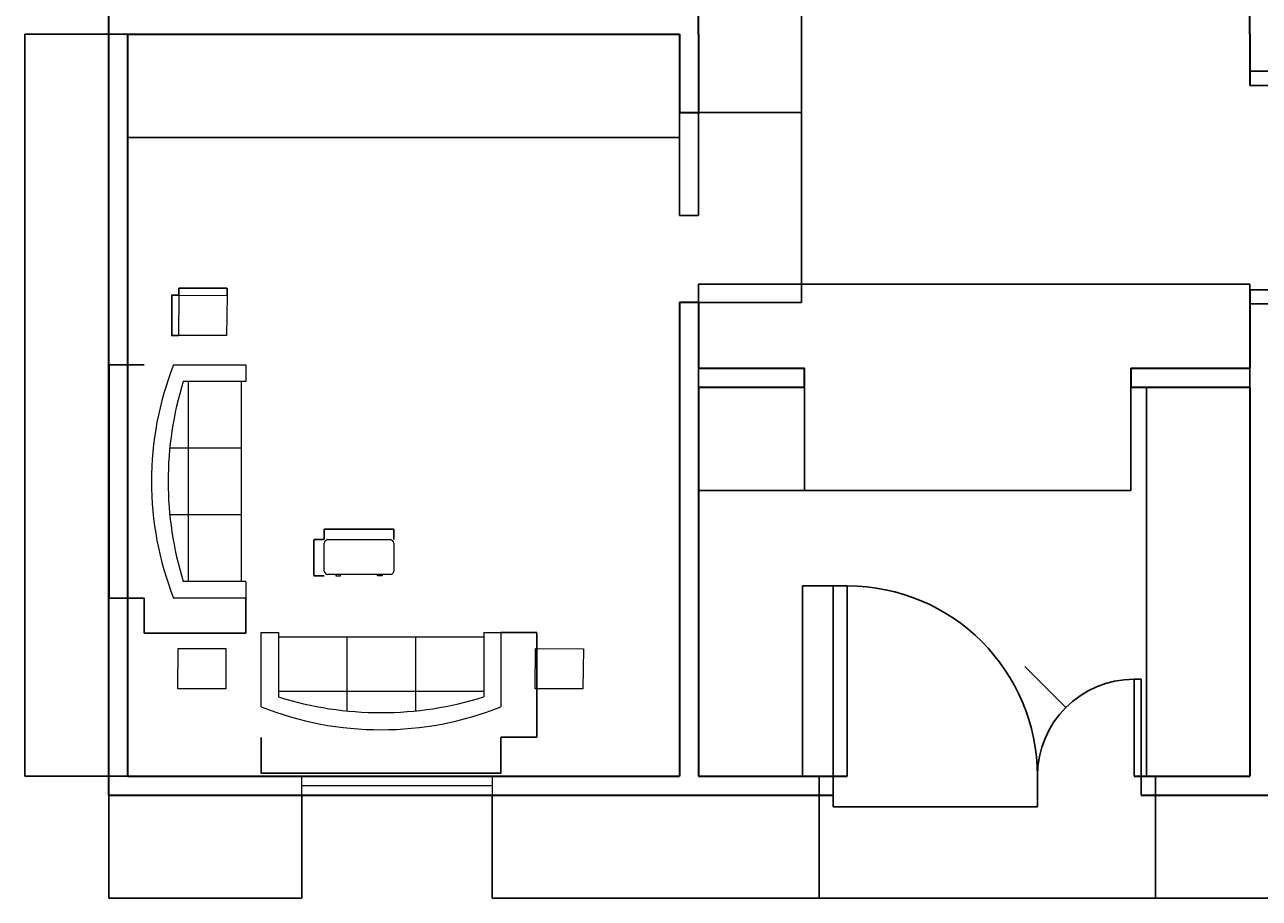
# Model space of a CAD drawing. Units: millimetres. Extents: x 1426 to 11512, y -8522 to 2664.
# Tile 1 of 4: x 1426 to 7919, y -8522 to -3929. Entities that reach past the tile are written whole.
import ezdxf

# ---------------------------------------------------------------- set-up
doc = ezdxf.new("R2010")
doc.units = ezdxf.units.MM
for name, color, linetype, lineweight in [('A-ANNO-DIMS', 2, 'Continuous', 18), ('A-DOOR', 3, 'Continuous', 25), ('A-FURN', 8, 'Continuous', 18), ('A-GLAZ', 4, 'Continuous', 18), ('A-WALL', 7, 'Continuous', 35)]:
    doc.layers.add(name, color=color, linetype=linetype, lineweight=lineweight)
doc.styles.get("Standard").update_dxf_attribs({"font": 'arial.ttf'})
doc.dimstyles.get("Standard").update_dxf_attribs({"dimtxt": 0.18, "dimasz": 0.18, "dimexe": 0.18, "dimexo": 0.0625, "dimgap": 0.09, "dimtad": 0, "dimtih": 1, "dimtoh": 1, "dimdec": 4, "dimzin": 0, "dimdsep": 46, "dimtxsty": 'Standard', "dimcen": 0.09, "dimadec": 0, "dimazin": 0, "dimtfac": 1, "dimtdec": 4, "dimtofl": 0, "dimtmove": 0, "dimatfit": 3, "dimfxl": 1, "dimtolj": 1, "dimtzin": 0, "dimarcsym": 0})

# ---------------------------------------------------------------- blocks, each defined once
blk = doc.blocks.new('Sofa - Roundback 7 ft.')
for p, q in [((-12.00002, -32.44210000000393), (-12.00003, -6.597100000003898)), ((11.99996999999999, -32.44210000000393), (11.99997999999999, -6.597100000003898)), ((-36.000027, -34.00000000000395), (-36.000027, -11.46960000000396)), ((35.99997999999999, -34.00000000000395), (35.99997999999999, -11.46960000000396)), ((-35.999844, -13.38190000000397), (35.99979999999999, -13.38190000000397)), ((-36.000027, -32.44210000000393), (35.99997999999999, -32.44210000000393))]:
    blk.add_line(p, q)
for points in [[(-36.000027, -34.00000000000395), (-42.000027, -34.00000000000395), (-42.000027, -8.000000000003944)], [(41.99997999999999, -8.000000000003944), (41.99997999999999, -34.00000000000395), (35.99997999999999, -34.00000000000395)]]:
    blk.add_lwpolyline(points)
for centre, radius, start, end in [((0, -114.2500000000039), 114.2500000000039, 68.43141000000072, 111.5686000000006), ((-1.00000000032e-05, -127.1968000000039), 121.1967999999973, 72.72032999999948, 107.2797000000005)]:
    blk.add_arc(centre, radius, start, end)
blk = doc.blocks.new('Desk - 30 x 60 in.')
for p, q in [((-26.999995, 0), (26.999995, 0)), ((-29.999995, -27), (-29.999995, -3)), ((29.999995, -3), (29.999995, -27)), ((26.999995, -30), (-26.999995, -30)), ((-20.000005, -30), (-20.000005, -31)), ((-20.000005, -31), (-16.000005, -31)), ((-16.000005, -31), (-16.000005, -30)), ((15.999995, -31), (15.999995, -30)), ((19.999995, -31), (15.999995, -31)), ((19.999995, -30), (19.999995, -31))]:
    blk.add_line(p, q)
for centre, radius, start, end in [((-26.499995, -3.5), 3.535534000004229, 98.1300999999916, 171.8698999999352), ((26.499995, -3.5), 3.535533999997753, 8.130102000022115, 81.8698999999439), ((-26.499995, -26.5), 3.535534000000845, 188.1301000000653, 261.8699000000085), ((26.499995, -26.5), 3.535534000004826, 278.1301000000561, 351.8698999999439)]:
    blk.add_arc(centre, radius, start, end)
blk = doc.blocks.new('DOOR-SINGLE-1000')
for p, q in [((-0.0002449408875691, 999.9999577541435), (-0.0002449408875691, 1099.999957754143)), ((-0.0002449408875691, 1099.999957754143), (74.19975505911316, 1099.999957754143)), ((74.19975505911316, 1099.999957754143), (74.19975505911316, 999.9999577541435)), ((1148.399755059116, 999.999957754143), (1148.399755059116, 1099.999957754143)), ((1148.399755059116, 1099.999957754143), (1222.599755059116, 1099.999957754143)), ((1222.599755059116, 1099.999957754143), (1222.599755059116, 999.9999577541435)), ((74.19975505911316, 999.9999577541435), (-0.0002449408875691, 999.9999577541435)), ((74.19975505911316, 999.9999577541435), (148.3997550591139, 999.9999577541435)), ((74.19975505911316, -4.22458564344e-05), (74.19975505911316, 999.9999577541435)), ((148.3997550591139, 999.9999577541435), (148.3997550591139, -4.22458564344e-05)), ((1222.599755059116, 999.999957754143), (1148.399755059116, 999.999957754143)), ((148.3997550591139, -4.22458564344e-05), (74.19975505911316, -4.22458564344e-05))]:
    blk.add_line(p, q)
blk.add_arc((148.3997550591157, 999.9999577541435), 999.9999999999998, 270, 0)
blk = doc.blocks.new('DOOR-LEAF-1000')
for p, q in [((999.9997662421769, 74.19984207478274), (-0.0002337578230254, 74.19984207478274)), ((-0.0002337578230254, 74.19984207478274), (-0.0002337578230254, -0.0001579252179909)), ((999.9997662421769, -0.0001579252179909), (999.9997662421769, 74.19984207478274)), ((-0.0002337578230254, -0.0001579252179909), (999.9997662421769, -0.0001579252179909))]:
    blk.add_line(p, q)
blk.add_arc((999.9997662421769, 74.19984207478456), 999.9999999999998, 90, 180)
blk = doc.blocks.new('WIN-1000')
for p, q in [((-0.0003881192678818, 99.99995775414573), (999.999611880732, 99.99995775414573)), ((-0.0003881192678818, -4.22458542744e-05), (-0.0003881192678818, 99.99995775414573)), ((999.999611880732, 99.99995775414573), (999.999611880732, -4.22458542744e-05)), ((-0.0003881192678818, 49.99995775414572), (999.999611880732, 49.99995775414572)), ((999.999611880732, -4.22458542744e-05), (-0.0003881192678818, -4.22458542744e-05))]:
    blk.add_line(p, q)
blk = doc.blocks.new('TABLE-END')
for p, q in [((0.5765397481395667, 0.4802073471801123), (1.381469779128565, 211.490897786076)), ((1.381469779128565, 211.490897786076), (253.6387314006142, 210.5286268935834)), ((253.6387314006142, 210.5286268935834), (250.8785212126982, -0.4746048534607326)), ((250.8785212126982, -0.4746048534607326), (0.5765397481395667, 0.4802073471801123))]:
    blk.add_line(p, q)
blk = doc.blocks.new('*D16')
at = {"layer": 'A-ANNO-DIMS', "color": 0, "lineweight": -2, "transparency": 16777216}
for p, q in [((2237.041557626602, -5351.488836398402), (2237.041557626602, -5313.41200765053)), ((2237.221557626601, -5313.59200765053), (2362.245736672484, -5313.59200765053)), ((2489.923749279077, -5313.59200765053), (2364.899570233193, -5313.59200765053)), ((2490.103749279076, -5351.488836398402), (2490.103749279076, -5313.41200765053))]:
    blk.add_line(p, q, dxfattribs=at)
at = {"layer": 'A-ANNO-DIMS', "color": 0, "transparency": 16777216}
for points in [[(2237.221557626601, -5313.562007650531), (2237.221557626601, -5313.622007650531), (2237.041557626602, -5313.59200765053)], [(2489.923749279077, -5313.562007650531), (2489.923749279077, -5313.622007650531), (2490.103749279076, -5313.59200765053)]]:
    blk.add_solid(points, dxfattribs=at)
at = {"layer": 'Defpoints', "color": 0, "transparency": 16777216}
for p in [(2490.103749279076, -5313.59200765053), (2237.041557626602, -5351.551336398402), (2490.103749279076, -5351.551336398402)]:
    blk.add_point(p, dxfattribs=at)
at = {"layer": 'A-ANNO-DIMS', "color": 0, "transparency": 16777216, "insert": (2363.572653452838, -5313.59200765053), "char_height": 0.18, "attachment_point": 5}
blk.add_mtext('\\A1;END TABLE 253 TYP.', dxfattribs=at)
blk = doc.blocks.new('*D17')
at = {"layer": 'A-ANNO-DIMS', "color": 0, "lineweight": -2, "transparency": 16777216}
for p, q in [((2236.979057626602, -5351.551336398404), (2198.902228878733, -5351.551336398404)), ((2199.082228878732, -5351.731336398405), (2199.082228878732, -5457.35365797738)), ((2199.082228878732, -5563.33683903794), (2199.082228878732, -5457.714517458963)), ((2236.979057626602, -5563.516839037941), (2198.902228878733, -5563.516839037941))]:
    blk.add_line(p, q, dxfattribs=at)
at = {"layer": 'A-ANNO-DIMS', "color": 0, "transparency": 16777216}
for points in [[(2199.052228878732, -5351.731336398405), (2199.112228878732, -5351.731336398405), (2199.082228878732, -5351.551336398404)], [(2199.052228878732, -5563.33683903794), (2199.112228878732, -5563.33683903794), (2199.082228878732, -5563.516839037941)]]:
    blk.add_solid(points, dxfattribs=at)
at = {"layer": 'Defpoints', "color": 0, "transparency": 16777216}
for p in [(2199.082228878732, -5351.551336398404), (2237.041557626602, -5351.551336398404), (2237.041557626602, -5563.516839037941)]:
    blk.add_point(p, dxfattribs=at)
at = {"layer": 'A-ANNO-DIMS', "color": 0, "transparency": 16777216, "insert": (2199.08222887873, -5457.534087718172), "char_height": 0.18, "attachment_point": 5}
blk.add_mtext('\\A1;212 TYP.', dxfattribs=at)
blk = doc.blocks.new('*D18')
at = {"layer": 'A-ANNO-DIMS', "color": 0, "lineweight": -2, "transparency": 16777216}
for p, q in [((2053.688910879819, -5716.972741680017), (1869.607763812478, -5716.972741680017)), ((1869.787763812478, -5717.152741680017), (1869.787763812478, -6330.001767602539)), ((1869.787763812478, -6943.217055462304), (1869.787763812478, -6330.368029539783)), ((2053.688910879819, -6943.397055462305), (1869.607763812478, -6943.397055462305))]:
    blk.add_line(p, q, dxfattribs=at)
at = {"layer": 'A-ANNO-DIMS', "color": 0, "transparency": 16777216}
for points in [[(1869.757763812478, -5717.152741680017), (1869.817763812478, -5717.152741680017), (1869.787763812478, -5716.972741680017)], [(1869.757763812478, -6943.217055462304), (1869.817763812478, -6943.217055462304), (1869.787763812478, -6943.397055462305)]]:
    blk.add_solid(points, dxfattribs=at)
at = {"layer": 'Defpoints', "color": 0, "transparency": 16777216}
for p in [(1869.787763812478, -5716.972741680017), (2053.751410879819, -5716.972741680017), (2053.751410879819, -6943.397055462305)]:
    blk.add_point(p, dxfattribs=at)
at = {"layer": 'A-ANNO-DIMS', "color": 0, "transparency": 16777216, "insert": (1869.787763812475, -6330.184898571159), "char_height": 0.18, "attachment_point": 5}
blk.add_mtext('\\A1;SOFA 1226', dxfattribs=at)
blk = doc.blocks.new('*D19')
at = {"layer": 'A-ANNO-DIMS', "color": 0, "lineweight": -2, "transparency": 16777216}
for p, q in [((2053.751410879818, -6943.4595554623), (2053.751410879818, -7127.540702529643)), ((2589.095269586896, -6943.4595554623), (2589.095269586896, -7127.540702529643)), ((2053.931410879818, -7127.360702529642), (2321.133817723125, -7127.360702529642)), ((2588.915269586896, -7127.360702529642), (2321.712862743589, -7127.360702529642))]:
    blk.add_line(p, q, dxfattribs=at)
at = {"layer": 'A-ANNO-DIMS', "color": 0, "transparency": 16777216}
for points in [[(2053.931410879818, -7127.330702529643), (2053.931410879818, -7127.390702529644), (2053.751410879818, -7127.360702529642)], [(2588.915269586896, -7127.330702529643), (2588.915269586896, -7127.390702529644), (2589.095269586896, -7127.360702529642)]]:
    blk.add_solid(points, dxfattribs=at)
at = {"layer": 'Defpoints', "color": 0, "transparency": 16777216}
for p in [(2053.751410879818, -6943.3970554623), (2589.095269586896, -6943.3970554623), (2053.751410879818, -7127.360702529642)]:
    blk.add_point(p, dxfattribs=at)
at = {"layer": 'A-ANNO-DIMS', "color": 0, "transparency": 16777216, "insert": (2321.423340233357, -7127.360702529642), "char_height": 0.18, "attachment_point": 5}
blk.add_mtext('\\A1;535', dxfattribs=at)
blk = doc.blocks.new('*D20')
at = {"layer": 'A-ANNO-DIMS', "color": 0, "lineweight": -2, "transparency": 16777216}
for p, q in [((2670.058380604727, -7675.536986969425), (2670.058380604727, -7864.771040374122)), ((3930.835403302701, -7675.536986969425), (3930.835403302701, -7864.771040374122)), ((2670.238380604727, -7864.591040374121), (3299.728672308421, -7864.591040374121)), ((3930.655403302701, -7864.591040374121), (3301.165111599007, -7864.591040374121))]:
    blk.add_line(p, q, dxfattribs=at)
at = {"layer": 'A-ANNO-DIMS', "color": 0, "transparency": 16777216}
for points in [[(2670.238380604727, -7864.561040374121), (2670.238380604727, -7864.621040374121), (2670.058380604727, -7864.591040374121)], [(3930.655403302701, -7864.561040374121), (3930.655403302701, -7864.621040374121), (3930.835403302701, -7864.591040374121)]]:
    blk.add_solid(points, dxfattribs=at)
at = {"layer": 'Defpoints', "color": 0, "transparency": 16777216}
for p in [(2670.058380604727, -7675.474486969425), (3930.835403302701, -7675.474486969425), (2670.058380604727, -7864.591040374121)]:
    blk.add_point(p, dxfattribs=at)
at = {"layer": 'A-ANNO-DIMS', "color": 0, "transparency": 16777216, "insert": (3300.446891953714, -7864.591040374121), "char_height": 0.18, "attachment_point": 5}
blk.add_mtext('\\A1;SOFA 1261', dxfattribs=at)
blk = doc.blocks.new('*D21')
at = {"layer": 'A-ANNO-DIMS', "color": 0, "lineweight": -2, "transparency": 16777216}
for p, q in [((3930.897903302703, -7125.13540063901), (4120.131956707401, -7125.13540063901)), ((4119.9519567074, -7125.31540063901), (4119.9519567074, -7400.123040666429)), ((4119.9519567074, -7675.294486969429), (4119.9519567074, -7400.486846942008)), ((3930.897903302703, -7675.474486969429), (4120.131956707401, -7675.474486969429))]:
    blk.add_line(p, q, dxfattribs=at)
at = {"layer": 'A-ANNO-DIMS', "color": 0, "transparency": 16777216}
for points in [[(4119.9219567074, -7125.31540063901), (4119.9819567074, -7125.31540063901), (4119.9519567074, -7125.13540063901)], [(4119.9219567074, -7675.294486969429), (4119.9819567074, -7675.294486969429), (4119.9519567074, -7675.474486969429)]]:
    blk.add_solid(points, dxfattribs=at)
at = {"layer": 'Defpoints', "color": 0, "transparency": 16777216}
for p in [(3930.835403302703, -7125.13540063901), (3930.835403302703, -7675.474486969429), (4119.9519567074, -7675.474486969429)]:
    blk.add_point(p, dxfattribs=at)
at = {"layer": 'A-ANNO-DIMS', "color": 0, "transparency": 16777216, "insert": (4119.951956707398, -7400.304943804218), "char_height": 0.18, "attachment_point": 5}
blk.add_mtext('\\A1;550', dxfattribs=at)
blk = doc.blocks.new('*D26')
at = {"layer": 'A-ANNO-DIMS', "color": 0, "lineweight": -2, "transparency": 16777216}
for p, q in [((5677.730172282599, -7879.117542245857), (5677.730172282599, -8040.365042245856)), ((6751.930172282602, -7879.117542245857), (6751.930172282602, -8040.365042245856)), ((5677.910172282599, -8040.185042245855), (6213.405213210294, -8040.185042245855)), ((6751.750172282601, -8040.185042245855), (6216.255131354905, -8040.185042245855))]:
    blk.add_line(p, q, dxfattribs=at)
at = {"layer": 'A-ANNO-DIMS', "color": 0, "transparency": 16777216}
for points in [[(5677.910172282599, -8040.155042245855), (5677.910172282599, -8040.215042245856), (5677.730172282599, -8040.185042245855)], [(6751.750172282601, -8040.155042245855), (6751.750172282601, -8040.215042245856), (6751.930172282602, -8040.185042245855)]]:
    blk.add_solid(points, dxfattribs=at)
at = {"layer": 'Defpoints', "color": 0, "transparency": 16777216}
for p in [(5677.730172282599, -7879.055042245856), (6751.930172282602, -7879.055042245856), (6751.930172282602, -8040.185042245855)]:
    blk.add_point(p, dxfattribs=at)
at = {"layer": 'A-ANNO-DIMS', "color": 0, "transparency": 16777216, "insert": (6214.830172282599, -8040.185042245855), "char_height": 0.18, "attachment_point": 5}
blk.add_mtext('\\A1;DOOR LEAF 1074 TYP.', dxfattribs=at)
blk = doc.blocks.new('*D27')
at = {"layer": 'A-ANNO-DIMS', "color": 0, "lineweight": -2, "transparency": 16777216}
for p, q in [((5677.667672282598, -6879.055042245861), (5516.420172282601, -6879.055042245861)), ((5516.600172282601, -6879.235042245861), (5516.600172282601, -7378.87313910807)), ((5516.600172282601, -7878.87504224586), (5516.600172282601, -7379.23694538365)), ((5677.6676722826, -7879.055042245861), (5516.420172282601, -7879.055042245861))]:
    blk.add_line(p, q, dxfattribs=at)
at = {"layer": 'A-ANNO-DIMS', "color": 0, "transparency": 16777216}
for points in [[(5516.570172282602, -6879.235042245861), (5516.630172282601, -6879.235042245861), (5516.600172282601, -6879.055042245861)], [(5516.570172282602, -7878.87504224586), (5516.630172282601, -7878.87504224586), (5516.600172282601, -7879.055042245861)]]:
    blk.add_solid(points, dxfattribs=at)
at = {"layer": 'Defpoints', "color": 0, "transparency": 16777216}
for p in [(5677.730172282599, -6879.055042245861), (5516.600172282601, -7879.055042245861), (5677.730172282601, -7879.055042245861)]:
    blk.add_point(p, dxfattribs=at)
at = {"layer": 'A-ANNO-DIMS', "color": 0, "transparency": 16777216, "insert": (5516.600172282599, -7379.055042245859), "char_height": 0.18, "attachment_point": 5}
blk.add_mtext('\\A1;1000 TYP.', dxfattribs=at)
blk = doc.blocks.new('*D36')
at = {"layer": 'A-ANNO-DIMS', "color": 0, "lineweight": -2, "transparency": 16777216}
for p, q in [((3001.124611822948, -6636.252036484484), (3001.124611822948, -6581.182263887985)), ((3001.304611822947, -6581.362263887985), (3183.637237167347, -6581.362263887985)), ((3367.293095799605, -6581.362263887985), (3184.960470455205, -6581.362263887985)), ((3367.473095799605, -6636.252036484484), (3367.473095799605, -6581.182263887985))]:
    blk.add_line(p, q, dxfattribs=at)
at = {"layer": 'A-ANNO-DIMS', "color": 0, "transparency": 16777216}
for points in [[(3001.304611822947, -6581.332263887985), (3001.304611822947, -6581.392263887984), (3001.124611822948, -6581.362263887985)], [(3367.293095799605, -6581.332263887985), (3367.293095799605, -6581.392263887984), (3367.473095799605, -6581.362263887985)]]:
    blk.add_solid(points, dxfattribs=at)
at = {"layer": 'Defpoints', "color": 0, "transparency": 16777216}
for p in [(3367.473095799605, -6581.362263887985), (3001.124611822948, -6636.314536484483), (3367.473095799605, -6636.314536484483)]:
    blk.add_point(p, dxfattribs=at)
at = {"layer": 'A-ANNO-DIMS', "color": 0, "transparency": 16777216, "insert": (3184.298853811276, -6581.362263887985), "char_height": 0.18, "attachment_point": 5}
blk.add_mtext('\\A1;DESK 366', dxfattribs=at)
blk = doc.blocks.new('*D37')
at = {"layer": 'A-ANNO-DIMS', "color": 0, "lineweight": -2, "transparency": 16777216}
for p, q in [((3001.062111822948, -6636.314536484488), (2945.992339226451, -6636.314536484488)), ((2946.172339226451, -6636.494536484488), (2946.172339226451, -6730.772674135775)), ((2946.172339226451, -6825.414618062641), (2946.172339226451, -6731.136480411355)), ((3001.062111822948, -6825.594618062641), (2945.992339226451, -6825.594618062641))]:
    blk.add_line(p, q, dxfattribs=at)
at = {"layer": 'A-ANNO-DIMS', "color": 0, "transparency": 16777216}
for points in [[(2946.142339226451, -6636.494536484488), (2946.202339226451, -6636.494536484488), (2946.172339226451, -6636.314536484488)], [(2946.142339226451, -6825.414618062641), (2946.202339226451, -6825.414618062641), (2946.172339226451, -6825.594618062641)]]:
    blk.add_solid(points, dxfattribs=at)
at = {"layer": 'Defpoints', "color": 0, "transparency": 16777216}
for p in [(2946.172339226451, -6636.314536484488), (3001.124611822949, -6636.314536484488), (3001.124611822949, -6825.594618062641)]:
    blk.add_point(p, dxfattribs=at)
at = {"layer": 'A-ANNO-DIMS', "color": 0, "transparency": 16777216, "insert": (2946.172339226448, -6730.954577273563), "char_height": 0.18, "attachment_point": 5}
blk.add_mtext('\\A1;189', dxfattribs=at)
blk = doc.blocks.new('*D40')
at = {"layer": 'A-ANNO-DIMS', "color": 0, "lineweight": -2, "transparency": 16777216}
for p, q in [((1968.871984, -3979.117542), (1968.871984, -4521.735042)), ((4868.871984, -3979.117542), (4868.871984, -4521.735042)), ((1969.051984, -4521.555042), (3418.511984000001, -4521.555042)), ((4868.691984, -4521.555042), (3419.231984, -4521.555042))]:
    blk.add_line(p, q, dxfattribs=at)
at = {"layer": 'A-ANNO-DIMS', "color": 0, "transparency": 16777216}
for points in [[(1969.051984, -4521.525042), (1969.051984, -4521.585041999999), (1968.871984, -4521.555042)], [(4868.691984, -4521.525042), (4868.691984, -4521.585041999999), (4868.871984, -4521.555042)]]:
    blk.add_solid(points, dxfattribs=at)
at = {"layer": 'Defpoints', "color": 0, "transparency": 16777216}
for p in [(1968.871984, -3979.055042), (4868.871984, -3979.055042), (1968.871984, -4521.555042)]:
    blk.add_point(p, dxfattribs=at)
at = {"layer": 'A-ANNO-DIMS', "color": 0, "transparency": 16777216, "insert": (3418.871984000001, -4521.555042), "char_height": 0.18, "attachment_point": 5}
blk.add_mtext('\\A1;2900', dxfattribs=at)
blk = doc.blocks.new('*D41')
at = {"layer": 'A-ANNO-DIMS', "color": 0, "lineweight": -2, "transparency": 16777216}
for p, q in [((4968.871984, -5835.356649000001), (4968.871984, -5292.739148999999)), ((4969.051984, -5292.919149), (6418.511984000002, -5292.919149)), ((7868.691984, -5292.919149), (6419.231983999999, -5292.919149)), ((7868.871984, -5835.356649000001), (7868.871984, -5292.739148999999))]:
    blk.add_line(p, q, dxfattribs=at)
at = {"layer": 'A-ANNO-DIMS', "color": 0, "transparency": 16777216}
for points in [[(4969.051984, -5292.889149), (4969.051984, -5292.949149), (4968.871984, -5292.919149)], [(7868.691984, -5292.889149), (7868.691984, -5292.949149), (7868.871984, -5292.919149)]]:
    blk.add_solid(points, dxfattribs=at)
at = {"layer": 'Defpoints', "color": 0, "transparency": 16777216}
for p in [(7868.871984, -5292.919149), (4968.871984, -5835.419149), (7868.871984, -5835.419149)]:
    blk.add_point(p, dxfattribs=at)
at = {"layer": 'A-ANNO-DIMS', "color": 0, "transparency": 16777216, "insert": (6418.871984, -5292.919149), "char_height": 0.18, "attachment_point": 5}
blk.add_mtext('\\A1;2900', dxfattribs=at)
blk = doc.blocks.new('*D45')
at = {"layer": 'A-ANNO-DIMS', "color": 0, "lineweight": -2, "transparency": 16777216}
for p, q in [((1968.809484000001, -3979.055042000002), (1426.191984, -3979.055042000002)), ((1426.371984, -3979.235042000002), (1426.371984000001, -5928.873077470671)), ((1426.371984000001, -7878.875042000003), (1426.371984000001, -5929.237006529334)), ((1968.809484000001, -7879.055042000003), (1426.191984000001, -7879.055042000003))]:
    blk.add_line(p, q, dxfattribs=at)
at = {"layer": 'A-ANNO-DIMS', "color": 0, "transparency": 16777216}
for points in [[(1426.341984, -3979.235042000002), (1426.401984, -3979.235042000002), (1426.371984, -3979.055042000002)], [(1426.341984000001, -7878.875042000003), (1426.401984000001, -7878.875042000003), (1426.371984000001, -7879.055042000003)]]:
    blk.add_solid(points, dxfattribs=at)
at = {"layer": 'Defpoints', "color": 0, "transparency": 16777216}
for p in [(1426.371984, -3979.055042000002), (1968.871984000001, -3979.055042000002), (1968.871984000001, -7879.055042000003)]:
    blk.add_point(p, dxfattribs=at)
at = {"layer": 'A-ANNO-DIMS', "color": 0, "transparency": 16777216, "insert": (1426.371983999999, -5929.055042000001), "char_height": 0.18, "attachment_point": 5}
blk.add_mtext('\\A1;3900', dxfattribs=at)
blk = doc.blocks.new('*D48')
at = {"layer": 'A-ANNO-DIMS', "color": 0, "lineweight": -2, "transparency": 16777216}
for p, q in [((4868.871984, -4390.061223), (4868.871984, -4932.678723)), ((4968.871984, -4390.061223), (4968.871984, -4932.678723)), ((4869.051984000001, -4932.498723), (4918.591915787176, -4932.498723)), ((4968.691984, -4932.498723), (4919.152052212824, -4932.498723))]:
    blk.add_line(p, q, dxfattribs=at)
at = {"layer": 'A-ANNO-DIMS', "color": 0, "transparency": 16777216}
for points in [[(4869.051984000001, -4932.468723), (4869.051984000001, -4932.528722999999), (4868.871984, -4932.498723)], [(4968.691984, -4932.468723), (4968.691984, -4932.528722999999), (4968.871984, -4932.498723)]]:
    blk.add_solid(points, dxfattribs=at)
at = {"layer": 'Defpoints', "color": 0, "transparency": 16777216}
for p in [(4868.871984, -4389.998723), (4968.871984, -4389.998723), (4868.871984, -4932.498723)]:
    blk.add_point(p, dxfattribs=at)
at = {"layer": 'A-ANNO-DIMS', "color": 0, "transparency": 16777216, "insert": (4918.871984, -4932.498723), "char_height": 0.18, "attachment_point": 5}
blk.add_mtext('\\A1;100', dxfattribs=at)
blk = doc.blocks.new('*D49')
at = {"layer": 'A-ANNO-DIMS', "color": 0, "lineweight": -2, "transparency": 16777216}
for p, q in [((7868.809484000005, -5835.419149000002), (7326.191984000006, -5835.419149000002)), ((7326.371984000006, -5835.599149000002), (7326.371984000008, -6857.055130970671)), ((7326.371984000008, -7878.875042000003), (7326.371984000008, -6857.419060029335)), ((7868.809484000005, -7879.055042000003), (7326.191984000008, -7879.055042000003))]:
    blk.add_line(p, q, dxfattribs=at)
at = {"layer": 'A-ANNO-DIMS', "color": 0, "transparency": 16777216}
for points in [[(7326.341984000007, -5835.599149000002), (7326.401984000006, -5835.599149000002), (7326.371984000006, -5835.419149000002)], [(7326.341984000008, -7878.875042000003), (7326.401984000007, -7878.875042000003), (7326.371984000008, -7879.055042000003)]]:
    blk.add_solid(points, dxfattribs=at)
at = {"layer": 'Defpoints', "color": 0, "transparency": 16777216}
for p in [(7326.371984000006, -5835.419149000002), (7868.871984000005, -5835.419149000002), (7868.871984000005, -7879.055042000003)]:
    blk.add_point(p, dxfattribs=at)
at = {"layer": 'A-ANNO-DIMS', "color": 0, "transparency": 16777216, "insert": (7326.371984000004, -6857.237095500003), "char_height": 0.18, "attachment_point": 5}
blk.add_mtext('\\A1;2043.6', dxfattribs=at)
blk = doc.blocks.new('*D50')
at = {"layer": 'A-ANNO-DIMS', "color": 0, "lineweight": -2, "transparency": 16777216}
for p, q in [((1868.871984, -7979.117542), (1868.871984000001, -8521.735042)), ((2883.980724, -7979.117542), (2883.980724000002, -8521.735041999998)), ((1869.051984000001, -8521.555042000002), (2375.988570916782, -8521.555042000002)), ((2883.800724000002, -8521.555041999998), (2376.864137083221, -8521.555042000002))]:
    blk.add_line(p, q, dxfattribs=at)
at = {"layer": 'A-ANNO-DIMS', "color": 0, "transparency": 16777216}
for points in [[(1869.051984000001, -8521.525041999997), (1869.051984000001, -8521.585042), (1868.871984000001, -8521.555042000002)], [(2883.800724000002, -8521.525041999997), (2883.800724000002, -8521.585041999999), (2883.980724000002, -8521.555041999998)]]:
    blk.add_solid(points, dxfattribs=at)
at = {"layer": 'Defpoints', "color": 0, "transparency": 16777216}
for p in [(1868.871984, -7979.055042), (2883.980724, -7979.055042), (1868.871984000001, -8521.555042000002)]:
    blk.add_point(p, dxfattribs=at)
at = {"layer": 'A-ANNO-DIMS', "color": 0, "transparency": 16777216, "insert": (2376.426354000002, -8521.555042000002), "char_height": 0.18, "attachment_point": 5}
blk.add_mtext('\\A1;1015.1', dxfattribs=at)
blk = doc.blocks.new('*D51')
at = {"layer": 'A-ANNO-DIMS', "color": 0, "lineweight": -2, "transparency": 16777216}
for p, q in [((3883.980724, -7979.117542), (3883.980723999998, -8521.735041999998)), ((5603.530172, -7979.117542), (5603.530171999998, -8521.735042000004)), ((3884.160723999997, -8521.555041999998), (4743.299615803545, -8521.555042000002)), ((5603.350171999998, -8521.555042000004), (4744.211280196451, -8521.555042000002))]:
    blk.add_line(p, q, dxfattribs=at)
at = {"layer": 'A-ANNO-DIMS', "color": 0, "transparency": 16777216}
for points in [[(3884.160723999997, -8521.525041999997), (3884.160723999997, -8521.585041999999), (3883.980723999998, -8521.555041999998)], [(5603.350171999998, -8521.525042000003), (5603.350171999998, -8521.585042000002), (5603.530171999998, -8521.555042000004)]]:
    blk.add_solid(points, dxfattribs=at)
at = {"layer": 'Defpoints', "color": 0, "transparency": 16777216}
for p in [(3883.980724, -7979.055042), (5603.530172, -7979.055042), (3883.980723999998, -8521.555041999998)]:
    blk.add_point(p, dxfattribs=at)
at = {"layer": 'A-ANNO-DIMS', "color": 0, "transparency": 16777216, "insert": (4743.755447999998, -8521.555042000002), "char_height": 0.18, "attachment_point": 5}
blk.add_mtext('\\A1;1719.5', dxfattribs=at)
blk = doc.blocks.new('*D52')
at = {"layer": 'A-ANNO-DIMS', "color": 0, "lineweight": -2, "transparency": 16777216}
for p, q in [((5603.530172, -7979.117542), (5603.530172, -8521.735042)), ((7372.550530000001, -7979.117542), (7372.550530000001, -8521.735042)), ((5603.710172, -8521.555042000002), (6487.689866688949, -8521.555042000002)), ((7372.370530000001, -8521.555042000002), (6488.39083531105, -8521.555042000002))]:
    blk.add_line(p, q, dxfattribs=at)
at = {"layer": 'A-ANNO-DIMS', "color": 0, "transparency": 16777216}
for points in [[(5603.710172, -8521.525041999997), (5603.710172, -8521.585042), (5603.530172, -8521.555042000002)], [(7372.370530000001, -8521.525041999997), (7372.370530000001, -8521.585042), (7372.550530000001, -8521.555042000002)]]:
    blk.add_solid(points, dxfattribs=at)
at = {"layer": 'Defpoints', "color": 0, "transparency": 16777216}
for p in [(5603.530172, -7979.055042), (7372.550530000001, -7979.055042), (5603.530172, -8521.555042000002)]:
    blk.add_point(p, dxfattribs=at)
at = {"layer": 'A-ANNO-DIMS', "color": 0, "transparency": 16777216, "insert": (6488.040350999999, -8521.555042000002), "char_height": 0.18, "attachment_point": 5}
blk.add_mtext('\\A1;1769', dxfattribs=at)
blk = doc.blocks.new('*D53')
at = {"layer": 'A-ANNO-DIMS', "color": 0, "lineweight": -2, "transparency": 16777216}
for p, q in [((7372.550530000001, -7979.117542), (7372.550530000001, -8521.735042)), ((9121.359612, -7979.117542), (9121.359612, -8521.735041999998)), ((7372.730530000001, -8521.555042000002), (8246.49972993588, -8521.555042000002)), ((9121.179612, -8521.555041999998), (8247.41041206412, -8521.555042000002))]:
    blk.add_line(p, q, dxfattribs=at)
at = {"layer": 'A-ANNO-DIMS', "color": 0, "transparency": 16777216}
for points in [[(7372.730530000001, -8521.525042000001), (7372.730530000001, -8521.585042000002), (7372.550530000001, -8521.555042000002)], [(9121.179612, -8521.525041999997), (9121.179612, -8521.585041999999), (9121.359612, -8521.555041999998)]]:
    blk.add_solid(points, dxfattribs=at)
at = {"layer": 'Defpoints', "color": 0, "transparency": 16777216}
for p in [(7372.550530000001, -7979.055042), (9121.359612, -7979.055042), (7372.550530000001, -8521.555042000002)]:
    blk.add_point(p, dxfattribs=at)
at = {"layer": 'A-ANNO-DIMS', "color": 0, "transparency": 16777216, "insert": (8246.955071, -8521.555042000002), "char_height": 0.18, "attachment_point": 5}
blk.add_mtext('\\A1;1748.8', dxfattribs=at)
blk = doc.blocks.new('*D63')
at = {"layer": 'A-ANNO-DIMS', "color": 0, "lineweight": -2, "transparency": 16777216}
for p, q in [((5527.102308, -5835.481649), (5527.102308, -6378.099149)), ((7242.872174, -5835.481649), (7242.872174, -6378.099149)), ((5527.282308000001, -6377.919149), (6384.531899935881, -6377.919149)), ((7242.692174, -6377.919149), (6385.442582064121, -6377.919149))]:
    blk.add_line(p, q, dxfattribs=at)
at = {"layer": 'A-ANNO-DIMS', "color": 0, "transparency": 16777216}
for points in [[(5527.282308000001, -6377.889149000001), (5527.282308000001, -6377.949149), (5527.102308, -6377.919149)], [(7242.692174, -6377.889149000001), (7242.692174, -6377.949149), (7242.872174, -6377.919149)]]:
    blk.add_solid(points, dxfattribs=at)
at = {"layer": 'Defpoints', "color": 0, "transparency": 16777216}
for p in [(5527.102308, -5835.419149), (7242.872174, -5835.419149), (5527.102308, -6377.919149)]:
    blk.add_point(p, dxfattribs=at)
at = {"layer": 'A-ANNO-DIMS', "color": 0, "transparency": 16777216, "insert": (6384.987241000001, -6377.919149), "char_height": 0.18, "attachment_point": 5}
blk.add_mtext('\\A1;1715.8', dxfattribs=at)
blk = doc.blocks.new('*D64')
at = {"layer": 'A-ANNO-DIMS', "color": 0, "lineweight": -2, "transparency": 16777216}
for p, q in [((4968.871984, -5835.481649), (4968.871984, -6378.099149)), ((5527.102308, -5835.481649), (5527.102308, -6378.099149)), ((4969.051984, -6377.919149), (5247.594362916781, -6377.919149)), ((5526.922308, -6377.919149), (5248.37992908322, -6377.919149))]:
    blk.add_line(p, q, dxfattribs=at)
at = {"layer": 'A-ANNO-DIMS', "color": 0, "transparency": 16777216}
for points in [[(4969.051984, -6377.889149000001), (4969.051984, -6377.949149), (4968.871984, -6377.919149)], [(5526.922308, -6377.889149000001), (5526.922308, -6377.949149), (5527.102308, -6377.919149)]]:
    blk.add_solid(points, dxfattribs=at)
at = {"layer": 'Defpoints', "color": 0, "transparency": 16777216}
for p in [(4968.871984, -5835.419149), (5527.102308, -5835.419149), (4968.871984, -6377.919149)]:
    blk.add_point(p, dxfattribs=at)
at = {"layer": 'A-ANNO-DIMS', "color": 0, "transparency": 16777216, "insert": (5247.987146, -6377.919149), "char_height": 0.18, "attachment_point": 5}
blk.add_mtext('\\A1;558.2', dxfattribs=at)
blk = doc.blocks.new('*D65')
at = {"layer": 'A-ANNO-DIMS', "color": 0, "lineweight": -2, "transparency": 16777216}
for p, q in [((4968.934484000002, -4389.998723000001), (5511.551984000004, -4389.998723000001)), ((5511.371984000004, -4390.178723000001), (5511.371984000004, -4889.816819862211)), ((5511.371984000004, -5389.818723000001), (5511.371984000004, -4890.180626137791)), ((4968.934484000002, -5389.998723000001), (5511.551984000004, -5389.998723000001))]:
    blk.add_line(p, q, dxfattribs=at)
at = {"layer": 'A-ANNO-DIMS', "color": 0, "transparency": 16777216}
for points in [[(5511.341984000004, -4390.178723000001), (5511.401984000004, -4390.178723000001), (5511.371984000004, -4389.998723000001)], [(5511.341984000004, -5389.818723000001), (5511.401984000004, -5389.818723000001), (5511.371984000004, -5389.998723000001)]]:
    blk.add_solid(points, dxfattribs=at)
at = {"layer": 'Defpoints', "color": 0, "transparency": 16777216}
for p in [(4968.871984000003, -4389.998723000001), (4968.871984000003, -5389.998723000001), (5511.371984000004, -5389.998723000001)]:
    blk.add_point(p, dxfattribs=at)
at = {"layer": 'A-ANNO-DIMS', "color": 0, "transparency": 16777216, "insert": (5511.371984000002, -4889.998723000001), "char_height": 0.18, "attachment_point": 5}
blk.add_mtext('\\A1;1000', dxfattribs=at)
blk = doc.blocks.new('*D66')
at = {"layer": 'A-ANNO-DIMS', "color": 0, "lineweight": -2, "transparency": 16777216}
for p, q in [((4968.934484000002, -3879.055042000002), (5511.551984000004, -3879.055042000002)), ((5511.371984000004, -3879.235042000001), (5511.371984000004, -4134.344979362211)), ((5511.371984000004, -4389.818723000001), (5511.371984000004, -4134.708785637791)), ((4968.934484000002, -4389.998723000001), (5511.551984000004, -4389.998723000001))]:
    blk.add_line(p, q, dxfattribs=at)
at = {"layer": 'A-ANNO-DIMS', "color": 0, "transparency": 16777216}
for points in [[(5511.341984000004, -3879.235042000001), (5511.401984000004, -3879.235042000001), (5511.371984000004, -3879.055042000002)], [(5511.341984000004, -4389.818723000001), (5511.401984000004, -4389.818723000001), (5511.371984000004, -4389.998723000001)]]:
    blk.add_solid(points, dxfattribs=at)
at = {"layer": 'Defpoints', "color": 0, "transparency": 16777216}
for p in [(4968.871984000003, -3879.055042000002), (4968.871984000003, -4389.998723000001), (5511.371984000004, -4389.998723000001)]:
    blk.add_point(p, dxfattribs=at)
at = {"layer": 'A-ANNO-DIMS', "color": 0, "transparency": 16777216, "insert": (5511.371984000002, -4134.526882500001), "char_height": 0.18, "attachment_point": 5}
blk.add_mtext('\\A1;510.9', dxfattribs=at)
blk = doc.blocks.new('*D75')
at = {"layer": 'A-ANNO-DIMS', "color": 0, "lineweight": -2, "transparency": 16777216}
for p, q in [((6684.925151168825, -7303.552963368826), (6685.105151168825, -7303.552963368826)), ((6685.105151168825, -7303.552963368826), (6900.790963834764, -7519.238963724008)), ((7260.516728999999, -7879.055042000001), (7260.696729, -7879.055042000003)), ((7260.606728999999, -7879.145042000001), (7260.606729, -7878.965042000003))]:
    blk.add_line(p, q, dxfattribs=at)
at = {"layer": 'A-ANNO-DIMS', "color": 0, "transparency": 16777216}
blk.add_solid([(6900.812177047431, -7519.217750529802), (6900.769750622099, -7519.260176918213), (6900.918242999999, -7519.366243000002)], dxfattribs=at)
at = {"layer": 'Defpoints', "color": 0, "transparency": 16777216}
for p in [(6900.918242999999, -7519.366243000002), (7260.606729, -7879.055042000003)]:
    blk.add_point(p, dxfattribs=at)
at = {"layer": 'A-ANNO-DIMS', "color": 0, "transparency": 16777216, "insert": (6684.4453148796, -7303.552963368826), "char_height": 0.18, "attachment_point": 5}
blk.add_mtext('\\A1;R508.7', dxfattribs=at)

msp = doc.modelspace()

# ---------------------------------------------------------------- linework, layer by layer
at = {"layer": 'A-DOOR'}
for p, q in [((7260.606729054064, -7879.055042245856), (7260.606729054064, -7370.378485474394)), ((7260.606729054064, -7370.378485474394), (7298.350529566507, -7370.378485474394)), ((7298.350529566507, -7370.378485474394), (7298.350529566507, -7879.055042245856)), ((5603.530172282597, -7879.055042245856), (5603.530172282597, -7979.055042245857)), ((5677.730172282598, -7879.055042245856), (5603.530172282597, -7879.055042245856)), ((5603.530172282597, -7879.055042245856), (5603.530172282597, -7979.055042245857)), ((5677.730172282598, -7979.055042245857), (5677.730172282598, -7879.055042245856)), ((7298.350529566507, -7879.055042245856), (7260.606729054064, -7879.055042245856)), ((7298.350529566507, -7879.055042245856), (7298.350529566507, -7979.055042245857)), ((7372.550529566509, -7879.055042245856), (7298.350529566507, -7879.055042245856)), ((7372.550529566509, -7979.055042245857), (7372.550529566509, -7879.055042245856)), ((5603.530172282597, -7979.055042245857), (5677.730172282598, -7979.055042245857)), ((7298.350529566507, -7979.055042245857), (7372.550529566509, -7979.055042245857))]:
    msp.add_line(p, q, dxfattribs=at)
msp.add_arc((7260.606729054064, -7879.055042245856), 508.676556771463, 90, 180, dxfattribs=at)
at = {"layer": 'A-WALL'}
for p, q in [((1868.871984386818, -7979.055042245855), (1868.871984386818, 2120.944957754144)), ((4968.871984386819, -3979.055042245857), (4968.871984386819, -3879.055042245856)), ((7868.87198438682, -3979.055042245857), (7868.87198438682, -3879.055042245857)), ((1968.871984386817, -7879.055042245855), (1968.871984386817, -3979.055042245857)), ((1968.871984386818, -3979.055042245857), (4868.871984386819, -3979.055042245857)), ((4868.871984386819, -3979.055042245857), (4868.871984386819, -4389.998722661083)), ((4968.871984386819, -3979.055042245857), (4968.871984386819, -4389.998722661083)), ((7868.87198438682, -3979.055042245857), (7868.87198438682, -4248.045845388629)), ((4868.871984386818, -4389.998722661083), (4968.871984386819, -4389.998722661083)), ((7868.87198438682, -5322.245845388631), (7868.87198438682, -5735.419149207011)), ((4968.871984386819, -5389.998722661083), (4868.871984386819, -5389.998722661083)), ((4868.871984386819, -5389.998722661083), (4868.871984386818, -7879.055042245855)), ((4968.871984386819, -5389.998722661083), (4968.871984386819, -5735.419149207011)), ((4968.871984386819, -5735.419149207011), (5527.102308421279, -5735.419149207011)), ((5527.102308421279, -5835.419149207011), (5527.102308421279, -5735.419149207011)), ((7242.872173879179, -5735.419149207011), (7242.872173879179, -5835.419149207011)), ((7242.872173879179, -5735.419149207011), (7868.87198438682, -5735.419149207011)), ((4968.871984386819, -5835.419149207011), (5527.102308421279, -5835.419149207011)), ((4968.871984386819, -5835.419149207011), (4968.871984386819, -7879.055042245855)), ((7242.872173879179, -5835.419149207011), (7868.87198438682, -5835.419149207011)), ((7868.87198438682, -5835.419149207012), (7868.87198438682, -7879.055042245855)), ((1968.871984386817, -7879.055042245852), (4868.871984386818, -7879.055042245855)), ((4968.871984386819, -7879.055042245855), (5751.930172282599, -7879.055042245855)), ((7260.606729054064, -7879.055042245855), (7868.871984386818, -7879.055042245855)), ((1868.871984386818, -7979.055042245855), (5677.730172282599, -7979.055042245857)), ((7298.350529566508, -7979.055042245857), (10968.87198438681, -7979.055042245857))]:
    msp.add_line(p, q, dxfattribs=at)

# ---------------------------------------------------------------- block references
at = {"layer": 'A-DOOR', "extrusion": (0, 0, -1), "zscale": -1, "rotation": 269.9999999999998}
msp.add_blockref('DOOR-SINGLE-1000', (-8968.87194214096, -4173.846090329516), dxfattribs=at)
at = {"layer": 'A-DOOR', "rotation": 270.0000000000001}
msp.add_blockref('DOOR-LEAF-1000', (5677.730330207815, -6879.05527600368), dxfattribs=at)
at = {"layer": 'A-FURN'}
for p in [(2236.465017878462, -5563.042234184478), (4110.53600079253, -7420.361000000001)]:
    msp.add_blockref('TABLE-END', p, dxfattribs=at)
for p, xscale, yscale, zscale, rotation in [((2092.685525003568, -6330.184623828169), 14.60028660539031, 14.60028660539031, 14.60028660539031, 90), ((3300.446609515048, -7635.449810407902), 15.00924734614225, 15.00924734614225, 15.00924734614225, 180)]:
    msp.add_blockref('Sofa - Roundback 7 ft.', p, dxfattribs=dict(at, xscale=xscale, yscale=yscale, zscale=zscale, rotation=rotation))
at = {"layer": 'A-FURN', "xscale": 6.105809060777628, "yscale": 6.105809060777628, "zscale": 6.105809060777628}
msp.add_blockref('Desk - 30 x 60 in.', (3184.298853811274, -6636.314537178531), dxfattribs=at)
at = {"layer": 'A-FURN', "rotation": 180.2185617694751}
msp.add_blockref('TABLE-END', (2484.248244174426, -7208.866202230712), dxfattribs=at)
at = {"layer": 'A-GLAZ'}
msp.add_blockref('WIN-1000', (2883.981111855961, -7979.054999999998), dxfattribs=at)

# ---------------------------------------------------------------- dimensions: what is measured, and where the dimension line sits
at = {"layer": 'A-ANNO-DIMS'}
for base, p1, p2, angle, override, picture, middle in [((5511.371984000004, -4389.998723000001), (4968.871984, -3879.055042), (4968.871984, -4389.998723), 270, {"dimdec": 1, "dimlfac": 1, "dimrnd": 0, "dimzin": 0, "dimdsep": 46, "dimlunit": 2}, '*D66', (5511.371984000002, -4134.526882500001)), ((1426.371984, -3979.055042000002), (1968.871984, -7879.055042), (1968.871984, -3979.055042), 90, {"dimdec": 0, "dimlfac": 1, "dimrnd": 0, "dimzin": 0, "dimdsep": 46, "dimlunit": 2}, '*D45', (1426.371983999999, -5929.055042000001)), ((1968.871984, -4521.555042), (4868.871984, -3979.055042), (1968.871984, -3979.055042), 180, {"dimdec": 0, "dimlfac": 1, "dimrnd": 0, "dimzin": 0, "dimdsep": 46, "dimlunit": 2}, '*D40', (3418.871984000001, -4521.555042)), ((4868.871984, -4932.498723), (4968.871984, -4389.998723), (4868.871984, -4389.998723), 180, {"dimdec": 0, "dimlfac": 1, "dimrnd": 0, "dimzin": 0, "dimdsep": 46, "dimlunit": 2}, '*D48', (4918.871984, -4932.498723)), ((5511.371984000004, -5389.998723000001), (4968.871984, -4389.998723), (4968.871984, -5389.998723), 270, {"dimdec": 0, "dimlfac": 1, "dimrnd": 0, "dimzin": 0, "dimdsep": 46, "dimlunit": 2}, '*D65', (5511.371984000002, -4889.998723000001)), ((4968.871984, -6377.919149), (5527.102308, -5835.419149), (4968.871984, -5835.419149), 180, {"dimdec": 1, "dimlfac": 1, "dimrnd": 0, "dimzin": 0, "dimdsep": 46, "dimlunit": 2}, '*D64', (5247.987146, -6377.919149)), ((5527.102308, -6377.919149), (7242.872174, -5835.419149), (5527.102308, -5835.419149), 180, {"dimdec": 1, "dimlfac": 1, "dimrnd": 0, "dimzin": 0, "dimdsep": 46, "dimlunit": 2}, '*D63', (6384.987241000001, -6377.919149)), ((7326.371984000006, -5835.419149000002), (7868.871984, -7879.055042), (7868.871984, -5835.419149), 89.99999999999994, {"dimdec": 1, "dimlfac": 1, "dimrnd": 0, "dimzin": 0, "dimdsep": 46, "dimlunit": 2}, '*D49', (7326.371984000004, -6857.237095500003)), ((2946.172339226451, -6636.314536484488), (3001.124611822948, -6825.594618062638), (3001.124611822948, -6636.314536484483), 90, {"dimdec": 0, "dimlfac": 1, "dimrnd": 0, "dimzin": 0, "dimdsep": 46, "dimlunit": 2}, '*D37', (2946.172339226448, -6730.954577273563)), ((2053.751410879818, -7127.360702529642), (2589.095269586896, -6943.3970554623), (2053.751410879818, -6943.3970554623), 180, {"dimdec": 0, "dimlfac": 1, "dimrnd": 0, "dimzin": 0, "dimdsep": 46, "dimlunit": 2}, '*D19', (2321.423340233357, -7127.360702529642)), ((4119.9519567074, -7675.474486969429), (3930.835403302701, -7125.135400639007), (3930.835403302701, -7675.474486969425), 270, {"dimdec": 0, "dimlfac": 1, "dimrnd": 0, "dimzin": 0, "dimdsep": 46, "dimlunit": 2}, '*D21', (4119.951956707398, -7400.304943804218)), ((1868.871984000001, -8521.555042000002), (2883.980724, -7979.055042), (1868.871984, -7979.055042), 180.0000000000001, {"dimdec": 1, "dimlfac": 1, "dimrnd": 0, "dimzin": 0, "dimdsep": 46, "dimlunit": 2}, '*D50', (2376.426354000002, -8521.555042000002)), ((3883.980723999998, -8521.555041999998), (5603.530172, -7979.055042), (3883.980724, -7979.055042), 179.9999999999998, {"dimdec": 1, "dimlfac": 1, "dimrnd": 0, "dimzin": 0, "dimdsep": 46, "dimlunit": 2}, '*D51', (4743.755447999998, -8521.555042000002)), ((5603.530172, -8521.555042000002), (7372.550530000001, -7979.055042), (5603.530172, -7979.055042), 180, {"dimdec": 0, "dimlfac": 1, "dimrnd": 0, "dimzin": 0, "dimdsep": 46, "dimlunit": 2}, '*D52', (6488.040350999999, -8521.555042000002)), ((7372.550530000001, -8521.555042000002), (9121.359612, -7979.055042), (7372.550530000001, -7979.055042), 180.0000000000001, {"dimdec": 1, "dimlfac": 1, "dimrnd": 0, "dimzin": 0, "dimdsep": 46, "dimlunit": 2}, '*D53', (8246.955071, -8521.555042000002))]:
    dim = msp.add_linear_dim(base=base, p1=p1, p2=p2, angle=angle, dimstyle='Standard', override=override, dxfattribs=at)
    dim.commit()
    dim.dimension.update_dxf_attribs({"geometry": picture, "text_midpoint": middle})
for base, p1, p2, text, picture, middle in [((2490.103749279076, -5313.59200765053), (2237.041557626602, -5351.551336398402), (2490.103749279076, -5351.551336398402), 'END TABLE <> TYP.', '*D16', (2363.572653452838, -5313.59200765053)), ((3367.473095799605, -6581.362263887985), (3001.124611822948, -6636.314536484483), (3367.473095799605, -6636.314536484483), 'DESK <>', '*D36', (3184.298853811276, -6581.362263887985))]:
    dim = msp.add_linear_dim(base=base, p1=p1, p2=p2, text=text, dimstyle='Standard', override={"dimdec": 0, "dimlfac": 1, "dimrnd": 0, "dimzin": 0, "dimdsep": 46, "dimlunit": 2}, dxfattribs=at)
    dim.commit()
    dim.dimension.update_dxf_attribs({"geometry": picture, "text_midpoint": middle})
dim = msp.add_linear_dim(base=(7868.871984, -5292.919149), p1=(4968.871984, -5835.419149), p2=(7868.871984, -5835.419149), dimstyle='Standard', override={"dimdec": 0, "dimlfac": 1, "dimrnd": 0, "dimzin": 0, "dimdsep": 46, "dimlunit": 2}, dxfattribs=at)
dim.commit()
dim.dimension.update_dxf_attribs({"geometry": '*D41', "text_midpoint": (6418.871984, -5292.919149)})
for base, p1, p2, angle, text, picture, middle in [((2199.082228878732, -5351.551336398404), (2237.041557626602, -5563.516839037938), (2237.041557626602, -5351.551336398402), 90, '<> TYP.', '*D17', (2199.08222887873, -5457.534087718172)), ((1869.787763812478, -5716.972741680017), (2053.751410879818, -6943.3970554623), (2053.751410879818, -5716.972741680014), 90, 'SOFA <>', '*D18', (1869.787763812475, -6330.184898571159)), ((5516.600172282601, -7879.055042245861), (5677.730172282597, -6879.055042245856), (5677.730172282599, -7879.055042245856), 270.0000000000001, '<> TYP.', '*D27', (5516.600172282599, -7379.055042245859)), ((2670.058380604727, -7864.591040374121), (3930.835403302701, -7675.474486969425), (2670.058380604727, -7675.474486969425), 180, 'SOFA <>', '*D20', (3300.446891953714, -7864.591040374121)), ((6751.930172282602, -8040.185042245855), (5677.730172282599, -7879.055042245856), (6751.930172282602, -7879.055042245856), 4.85e-14, 'DOOR LEAF <> TYP.', '*D26', (6214.830172282599, -8040.185042245855))]:
    dim = msp.add_linear_dim(base=base, p1=p1, p2=p2, angle=angle, text=text, dimstyle='Standard', override={"dimdec": 0, "dimlfac": 1, "dimrnd": 0, "dimzin": 0, "dimdsep": 46, "dimlunit": 2}, dxfattribs=at)
    dim.commit()
    dim.dimension.update_dxf_attribs({"geometry": picture, "text_midpoint": middle})
dim = msp.add_radius_dim(center=(7260.606729, -7879.055042000003), mpoint=(6900.918242999999, -7519.366243000002), dimstyle='Standard', override={"dimdec": 1, "dimlfac": 1, "dimrnd": 0, "dimzin": 0, "dimdsep": 46, "dimlunit": 2}, dxfattribs=at)
dim.commit()
dim.dimension.update_dxf_attribs({"geometry": '*D75', "text_midpoint": (6684.4453148796, -7303.552963368826), "dimtype": 164})

doc.saveas('drawing.dxf')
